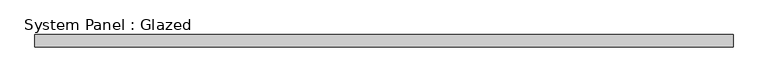
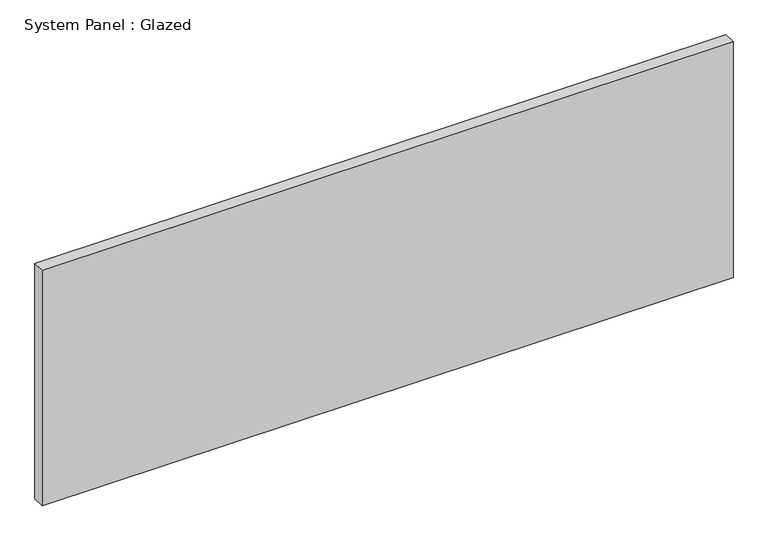
"""IFC4 building model written with IfcOpenShell, lengths in millimetres: plate geometry, System Panel : Glazed."""

from ifc_helpers import new_model, si_unit, origin, origin_with_axes, place, context, project, spatial, polyline, outline, extrude, source, transform, mapped, element, save


def system_panel_glazed_b12e8a87(model_context):
    return source(origin(), model_context, "Body", "SweptSolid", [
        extrude(outline(polyline([(713.3166667, 19.05), (-713.3166667, 19.05), (-713.3166667, 44.45), (713.3166667, 44.45), (713.3166667, 19.05)])), origin_with_axes(), (0.0, 0.0, 1.0), 514.35),
    ])


if __name__ == "__main__":
    model = new_model("IFC4")
    model_context = context("Model", 3, world=origin())
    ifc_project = project(units=[si_unit("LENGTHUNIT", "METRE", prefix="MILLI")], contexts=[model_context])
    site = spatial("IfcSite", under=ifc_project)
    building = spatial("IfcBuilding", under=site)
    placement = place(None, origin())
    system_panel_glazed_shape = system_panel_glazed_b12e8a87(model_context)
    element("IfcPlate", 1, ObjectType="System Panel : Glazed", at=placement, inside=building, context=model_context, shape_type="MappedRepresentation", body=[
        mapped(system_panel_glazed_shape, transform((0.0, 0.0, 0.0), x_axis=(1.0, 0.0, 0.0), y_axis=(0.0, 1.0, 0.0), z_axis=(0.0, 0.0, 1.0))),
    ])
    save(model, "model.ifc")

# Revit data of these elements
# Type "System Panel : Glazed"
#   Construction Type Id = "GSP4R"
#   Analytic Construction = "1/8 in Pilkington single glazing"
#   Visual Light Transmittance = 0.9
#   Solar Heat Gain Coefficient = 0.86
#   Heat Transfer Coefficient (U) = 1.18115 BTU/(h·ft²·°F)
# Element 1 (IfcPlate, "System Panel : Glazed")
#   Materials on its faces: "Glass"
# Materials
#   "Glass": class "Glass", colour RGB 0 128 192, transparency 0.75, Description = "Soda Lime Glass", Cost = 0
